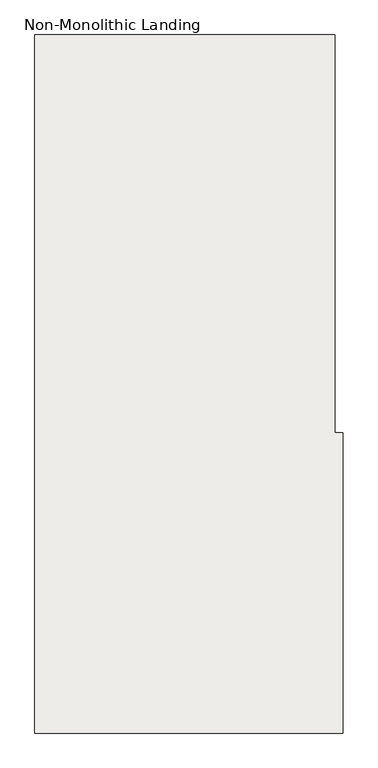
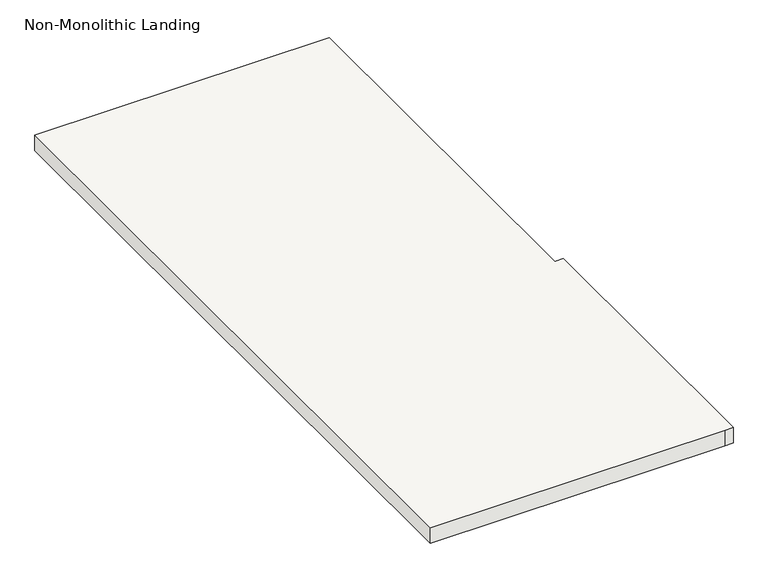
"""IFC4 building model written with IfcOpenShell, lengths in millimetres: slab geometry, Non-Monolithic Landing."""

from ifc_helpers import new_model, si_unit, origin, place, context, project, spatial, faceted_brep, source, transform, mapped, element, save


def non_monolithic_landing_6f6b2bb5(model_context):
    return source(origin(), model_context, "Body", "Brep", [
        faceted_brep([(-8810.2517085, 2919.0826226, 5475.8166667), (-8784.8517085, 2919.0826226, 5501.2166667), (-8784.8517085, 2004.6826226, 5501.2166667), (-8810.2517085, 2004.6826226, 5475.8166667), (-9699.2517085, 2919.0826226, 5520.2666667), (-9699.2517085, 792.0165128, 5520.2666667), (-8784.8517085, 792.0165128, 5520.2666667), (-8759.4517085, 792.0165128, 5520.2666667), (-8759.4517085, 1706.4165128, 5520.2666667), (-8784.8517085, 1706.4165128, 5520.2666667), (-8784.8517085, 2919.0826226, 5520.2666667), (-8810.2517085, 2004.6826226, 5469.4666667), (-8784.8517085, 2004.6826226, 5469.4666667), (-8784.8517085, 1706.4165128, 5469.4666667), (-8759.4517085, 1706.4165128, 5469.4666667), (-8759.4517085, 792.0165128, 5469.4666667), (-8784.8517085, 792.0165128, 5469.4666667), (-9699.2517085, 792.0165128, 5469.4666667), (-9699.2517085, 2919.0826226, 5469.4666667), (-8810.2517085, 2919.0826226, 5469.4666667)], [[[0, 1, 2, 3]], [[4, 5, 6, 7, 8, 9, 10]], [[11, 12, 13, 14, 15, 16, 17, 18, 19]], [[12, 11, 3, 2]], [[11, 19, 0, 3]], [[4, 10, 1, 0, 19, 18]], [[5, 4, 18, 17]], [[6, 5, 17, 16]], [[7, 6, 16, 15]], [[8, 7, 15, 14]], [[9, 8, 14, 13]], [[10, 9, 13, 12, 2, 1]]]),
    ])


if __name__ == "__main__":
    model = new_model("IFC4")
    model_context = context("Model", 3, world=origin())
    ifc_project = project(units=[si_unit("LENGTHUNIT", "METRE", prefix="MILLI")], contexts=[model_context])
    site = spatial("IfcSite", under=ifc_project)
    building = spatial("IfcBuilding", under=site)
    placement = place(None, origin())
    non_monolithic_landing_shape = non_monolithic_landing_6f6b2bb5(model_context)
    element("IfcSlab", 1, ObjectType="Non-Monolithic Landing", at=placement, inside=building, context=model_context, shape_type="MappedRepresentation", body=[
        mapped(non_monolithic_landing_shape, transform((0.0, 0.0, 0.0), x_axis=(1.0, 0.0, 0.0), y_axis=(0.0, 1.0, 0.0), z_axis=(0.0, 0.0, 1.0))),
    ])
    save(model, "model.ifc")
